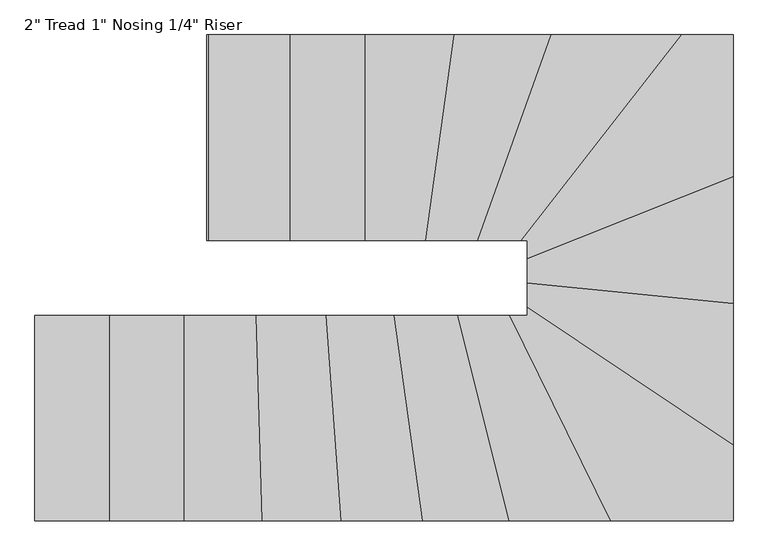
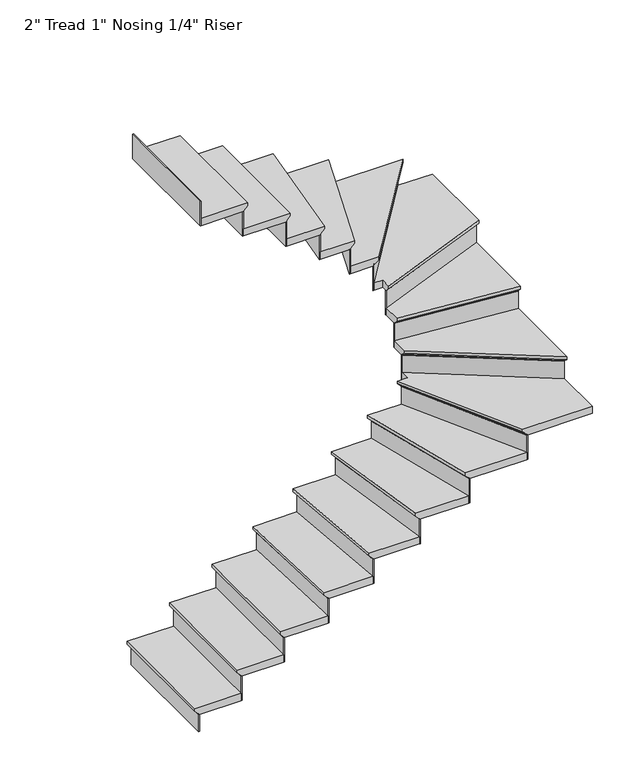
"""IFC4 building model written with IfcOpenShell, lengths in millimetres: stair flight geometry."""

from ifc_helpers import new_model, si_unit, origin, place, context, project, spatial, faceted_brep, source, transform, mapped, element, save


def stair_flight_f4c31f77(model_context):
    return source(origin(), model_context, "Body", "Brep", [
        faceted_brep([(-7679.0298583, 5178.9261204, 150.2833333), (-7679.0298583, 5178.9261204, 169.3333333), (-7679.0298583, 5948.2839473, 169.3333333), (-7679.0298583, 5948.2839473, 150.2833333), (-7653.6298583, 5178.9261204, 124.8833333), (-7653.6298583, 5948.2839473, 124.8833333), (-7374.2298583, 5178.9261204, 169.3333333), (-7374.2298583, 5948.2839473, 169.3333333), (-7653.6298583, 5948.2839473, 118.5333333), (-7374.2298583, 5948.2839473, 118.5333333), (-7374.2298583, 5178.9261204, 118.5333333), (-7653.6298583, 5178.9261204, 118.5333333)], [[[0, 1, 2, 3]], [[4, 0, 3, 5]], [[2, 1, 6, 7]], [[8, 9, 10, 11]], [[2, 7, 9, 8, 5, 3]], [[8, 11, 4, 5]], [[6, 1, 0, 4, 11, 10]], [[7, 6, 10, 9]]]),
        faceted_brep([(-7653.6298583, 5178.9261204, 118.5333333), (-7653.6298583, 5178.9261204, 0.0), (-7647.2798583, 5178.9261204, 0.0), (-7647.2798583, 5178.9261204, 118.5333333), (-7653.6298583, 5948.2839473, 118.5333333), (-7647.2798583, 5948.2839473, 118.5333333), (-7647.2798583, 5948.2839473, 0.0), (-7653.6298583, 5948.2839473, 0.0)], [[[0, 1, 2, 3]], [[4, 5, 6, 7]], [[1, 0, 4, 7]], [[2, 1, 7, 6]], [[3, 2, 6, 5]], [[0, 3, 5, 4]]]),
        faceted_brep([(-7374.2298583, 5178.9261204, 287.8666667), (-7374.2298583, 5178.9261204, 118.5333333), (-7367.8798583, 5178.9261204, 118.5333333), (-7367.8798583, 5178.9261204, 287.8666667), (-7374.2298583, 5948.2839473, 287.8666667), (-7367.8798583, 5948.2839473, 287.8666667), (-7367.8798583, 5948.2839473, 118.5333333), (-7374.2298583, 5948.2839473, 118.5333333)], [[[0, 1, 2, 3]], [[4, 5, 6, 7]], [[1, 0, 4, 7]], [[2, 1, 7, 6]], [[3, 2, 6, 5]], [[0, 3, 5, 4]]]),
        faceted_brep([(-7399.6298583, 5948.2839473, 338.6666667), (-7399.6298583, 5178.9261204, 338.6666667), (-7094.8298583, 5178.9261204, 338.6666667), (-7094.8298583, 5948.2839473, 338.6666667), (-7374.2298583, 5948.2839473, 287.8666667), (-7094.8298583, 5948.2839473, 287.8666667), (-7094.8298583, 5178.9261204, 287.8666667), (-7374.2298583, 5178.9261204, 287.8666667), (-7374.2298583, 5948.2839473, 294.2166667), (-7399.6298583, 5948.2839473, 319.6166667), (-7374.2298583, 5178.9261204, 294.2166667), (-7399.6298583, 5178.9261204, 319.6166667)], [[[0, 1, 2, 3]], [[4, 5, 6, 7]], [[0, 3, 5, 4, 8, 9]], [[4, 7, 10, 8]], [[2, 1, 11, 10, 7, 6]], [[3, 2, 6, 5]], [[11, 1, 0, 9]], [[10, 11, 9, 8]]]),
        faceted_brep([(-7094.8298583, 5178.9261204, 457.2), (-7094.8298583, 5178.9261204, 287.8666667), (-7088.4798583, 5178.9261204, 287.8666667), (-7088.4798583, 5178.9261204, 457.2), (-7094.8298583, 5948.2839473, 457.2), (-7088.4798583, 5948.2839473, 457.2), (-7088.4798583, 5948.2839473, 287.8666667), (-7094.8298583, 5948.2839473, 287.8666667)], [[[0, 1, 2, 3]], [[4, 5, 6, 7]], [[1, 0, 4, 7]], [[2, 1, 7, 6]], [[3, 2, 6, 5]], [[0, 3, 5, 4]]]),
        faceted_brep([(-7120.2298583, 5948.2839473, 508.0), (-7120.2298583, 5178.9261204, 508.0), (-6803.7593051, 5178.9261204, 508.0), (-6827.0770849, 5948.2839473, 508.0), (-7094.8298583, 5948.2839473, 457.2), (-6827.0770849, 5948.2839473, 457.2), (-6803.7593051, 5178.9261204, 457.2), (-7094.8298583, 5178.9261204, 457.2), (-7094.8298583, 5948.2839473, 463.55), (-7120.2298583, 5948.2839473, 488.95), (-7094.8298583, 5178.9261204, 463.55), (-7120.2298583, 5178.9261204, 488.95)], [[[0, 1, 2, 3]], [[4, 5, 6, 7]], [[0, 3, 5, 4, 8, 9]], [[4, 7, 10, 8]], [[2, 1, 11, 10, 7, 6]], [[3, 2, 6, 5]], [[11, 1, 0, 9]], [[10, 11, 9, 8]]]),
        faceted_brep([(-6803.7593051, 5178.9261204, 626.5333333), (-6803.7593051, 5178.9261204, 457.2), (-6797.4063893, 5178.9261204, 457.2), (-6797.4063893, 5178.9261204, 626.5333333), (-6827.0770849, 5948.2839473, 626.5333333), (-6820.7241691, 5948.2839473, 626.5333333), (-6820.7241691, 5948.2839473, 457.2), (-6827.0770849, 5948.2839473, 457.2)], [[[0, 1, 2, 3]], [[4, 5, 6, 7]], [[1, 0, 4, 7]], [[2, 1, 7, 6]], [[3, 2, 6, 5]], [[0, 3, 5, 4]]]),
        faceted_brep([(-6852.4887482, 5948.2839473, 677.3333333), (-6829.1709684, 5178.9261204, 677.3333333), (-6507.7862116, 5178.9261204, 677.3333333), (-6564.1374226, 5948.2839473, 677.3333333), (-6827.0770849, 5948.2839473, 626.5333333), (-6564.1374226, 5948.2839473, 626.5333333), (-6507.7862116, 5178.9261204, 626.5333333), (-6803.7593051, 5178.9261204, 626.5333333), (-6827.0770849, 5948.2839473, 632.8833333), (-6852.4887482, 5948.2839473, 658.2833333), (-6803.7593051, 5178.9261204, 632.8833333), (-6829.1709684, 5178.9261204, 658.2833333)], [[[0, 1, 2, 3]], [[4, 5, 6, 7]], [[0, 3, 5, 4, 8, 9]], [[4, 7, 10, 8]], [[2, 1, 11, 10, 7, 6]], [[3, 2, 6, 5]], [[11, 1, 0, 9]], [[10, 11, 9, 8]]]),
        faceted_brep([(-6507.7862116, 5178.9261204, 795.8666667), (-6507.7862116, 5178.9261204, 626.5333333), (-6501.4192013, 5178.9261204, 626.5333333), (-6501.4192013, 5178.9261204, 795.8666667), (-6564.1374226, 5948.2839473, 795.8666667), (-6557.7704123, 5948.2839473, 795.8666667), (-6557.7704123, 5948.2839473, 626.5333333), (-6564.1374226, 5948.2839473, 626.5333333)], [[[0, 1, 2, 3]], [[4, 5, 6, 7]], [[1, 0, 4, 7]], [[2, 1, 7, 6]], [[3, 2, 6, 5]], [[0, 3, 5, 4]]]),
        faceted_brep([(-6589.6054638, 5948.2839473, 846.6666667), (-6533.2542529, 5178.9261204, 846.6666667), (-6203.0012017, 5178.9261204, 846.6666667), (-6309.7716562, 5948.2839473, 846.6666667), (-6564.1374226, 5948.2839473, 795.8666667), (-6309.7716562, 5948.2839473, 795.8666667), (-6203.0012017, 5178.9261204, 795.8666667), (-6507.7862116, 5178.9261204, 795.8666667), (-6564.1374226, 5948.2839473, 802.2166667), (-6589.6054638, 5948.2839473, 827.6166667), (-6507.7862116, 5178.9261204, 802.2166667), (-6533.2542529, 5178.9261204, 827.6166667)], [[[0, 1, 2, 3]], [[4, 5, 6, 7]], [[0, 3, 5, 4, 8, 9]], [[4, 7, 10, 8]], [[2, 1, 11, 10, 7, 6]], [[3, 2, 6, 5]], [[11, 1, 0, 9]], [[10, 11, 9, 8]]]),
        faceted_brep([(-6203.0012017, 5178.9261204, 965.2), (-6203.0012017, 5178.9261204, 795.8666667), (-6196.5903443, 5178.9261204, 795.8666667), (-6196.5903443, 5178.9261204, 965.2), (-6309.7716562, 5948.2839473, 965.2), (-6303.3607989, 5948.2839473, 965.2), (-6303.3607989, 5948.2839473, 795.8666667), (-6309.7716562, 5948.2839473, 795.8666667)], [[[0, 1, 2, 3]], [[4, 5, 6, 7]], [[1, 0, 4, 7]], [[2, 1, 7, 6]], [[3, 2, 6, 5]], [[0, 3, 5, 4]]]),
        faceted_brep([(-6335.4150856, 5948.2839473, 1016.0), (-6228.6446311, 5178.9261204, 1016.0), (-5879.8397743, 5178.9261204, 1016.0), (-6073.0426446, 5948.2839473, 1016.0), (-6309.7716562, 5948.2839473, 965.2), (-6073.0426446, 5948.2839473, 965.2), (-5879.8397743, 5178.9261204, 965.2), (-6203.0012017, 5178.9261204, 965.2), (-6309.7716562, 5948.2839473, 971.55), (-6335.4150856, 5948.2839473, 996.95), (-6203.0012017, 5178.9261204, 971.55), (-6228.6446311, 5178.9261204, 996.95)], [[[0, 1, 2, 3]], [[4, 5, 6, 7]], [[0, 3, 5, 4, 8, 9]], [[4, 7, 10, 8]], [[2, 1, 11, 10, 7, 6]], [[3, 2, 6, 5]], [[11, 1, 0, 9]], [[10, 11, 9, 8]]]),
        faceted_brep([(-5879.8397743, 5178.9261204, 1134.5333333), (-5879.8397743, 5178.9261204, 965.2), (-5873.2926121, 5178.9261204, 965.2), (-5873.2926121, 5178.9261204, 1134.5333333), (-6073.0426446, 5948.2839473, 1134.5333333), (-6066.4954824, 5948.2839473, 1134.5333333), (-6066.4954824, 5948.2839473, 965.2), (-6073.0426446, 5948.2839473, 965.2)], [[[0, 1, 2, 3]], [[4, 5, 6, 7]], [[1, 0, 4, 7]], [[2, 1, 7, 6]], [[3, 2, 6, 5]], [[0, 3, 5, 4]]]),
        faceted_brep([(-6099.2312935, 5948.2839473, 1185.3333333), (-5906.0284232, 5178.9261204, 1185.3333333), (-5497.940126, 5178.9261204, 1185.3333333), (-5875.7797358, 5948.2839473, 1185.3333333), (-6073.0426446, 5948.2839473, 1134.5333333), (-5875.7797358, 5948.2839473, 1134.5333333), (-5497.940126, 5178.9261204, 1134.5333333), (-5879.8397743, 5178.9261204, 1134.5333333), (-6073.0426446, 5948.2839473, 1140.8833333), (-6099.2312935, 5948.2839473, 1166.2833333), (-5879.8397743, 5178.9261204, 1140.8833333), (-5906.0284232, 5178.9261204, 1166.2833333)], [[[0, 1, 2, 3]], [[4, 5, 6, 7]], [[0, 3, 5, 4, 8, 9]], [[4, 7, 10, 8]], [[2, 1, 11, 10, 7, 6]], [[3, 2, 6, 5]], [[11, 1, 0, 9]], [[10, 11, 9, 8]]]),
        faceted_brep([(-5497.940126, 5178.9261204, 1303.8666667), (-5497.940126, 5178.9261204, 1134.5333333), (-5490.8656748, 5178.9261204, 1134.5333333), (-5490.8656748, 5178.9261204, 1303.8666667), (-5875.7797358, 5948.2839473, 1303.8666667), (-5868.7052846, 5948.2839473, 1303.8666667), (-5868.7052846, 5948.2839473, 1134.5333333), (-5875.7797358, 5948.2839473, 1134.5333333)], [[[0, 1, 2, 3]], [[4, 5, 6, 7]], [[1, 0, 4, 7]], [[2, 1, 7, 6]], [[3, 2, 6, 5]], [[0, 3, 5, 4]]]),
        faceted_brep([(-5838.68475, 6008.9671044, 1354.6666667), (-5838.68475, 5948.2839473, 1354.6666667), (-5904.0775406, 5948.2839473, 1354.6666667), (-5526.2379307, 5178.9261204, 1354.6666667), (-5069.3269231, 5178.9261204, 1354.6666667), (-5069.3269231, 5494.6042749, 1354.6666667), (-5838.68475, 5948.2839473, 1303.8666667), (-5838.68475, 6008.9671044, 1303.8666667), (-5069.3269231, 5494.6042749, 1303.8666667), (-5069.3269231, 5178.9261204, 1303.8666667), (-5497.940126, 5178.9261204, 1303.8666667), (-5875.7797358, 5948.2839473, 1303.8666667), (-5497.940126, 5178.9261204, 1310.2166667), (-5875.7797358, 5948.2839473, 1310.2166667), (-5526.2379307, 5178.9261204, 1335.6166667), (-5904.0775406, 5948.2839473, 1335.6166667)], [[[0, 1, 2, 3, 4, 5]], [[6, 7, 8, 9, 10, 11]], [[1, 0, 7, 6]], [[11, 10, 12, 13]], [[5, 4, 9, 8]], [[0, 5, 8, 7]], [[14, 3, 2, 15]], [[12, 14, 15, 13]], [[4, 3, 14, 12, 10, 9]], [[2, 1, 6, 11, 13, 15]]]),
        faceted_brep([(-5069.3269231, 5494.6042749, 1473.2), (-5069.3269231, 5494.6042749, 1303.8666667), (-5069.3269231, 5502.242705, 1303.8666667), (-5069.3269231, 5502.242705, 1473.2), (-5838.68475, 6008.9671044, 1473.2), (-5838.68475, 6016.6055346, 1473.2), (-5838.68475, 6016.6055346, 1303.8666667), (-5838.68475, 6008.9671044, 1303.8666667)], [[[0, 1, 2, 3]], [[4, 5, 6, 7]], [[1, 0, 4, 7]], [[2, 1, 7, 6]], [[3, 2, 6, 5]], [[0, 3, 5, 4]]]),
        faceted_brep([(-5838.68475, 5978.4133839, 1524.0), (-5069.3269231, 5464.0505544, 1524.0), (-5069.3269231, 6017.5402175, 1524.0), (-5838.68475, 6094.2010538, 1524.0), (-5838.68475, 6008.9671044, 1473.2), (-5838.68475, 6094.2010538, 1473.2), (-5069.3269231, 6017.5402175, 1473.2), (-5069.3269231, 5494.6042749, 1473.2), (-5838.68475, 6008.9671044, 1479.55), (-5838.68475, 5978.4133839, 1504.95), (-5069.3269231, 5494.6042749, 1479.55), (-5069.3269231, 5464.0505544, 1504.95)], [[[0, 1, 2, 3]], [[4, 5, 6, 7]], [[0, 3, 5, 4, 8, 9]], [[4, 7, 10, 8]], [[2, 1, 11, 10, 7, 6]], [[3, 2, 6, 5]], [[11, 1, 0, 9]], [[10, 11, 9, 8]]]),
        faceted_brep([(-5069.3269231, 6017.5402175, 1642.5333333), (-5069.3269231, 6017.5402175, 1473.2), (-5069.3269231, 6023.9216631, 1473.2), (-5069.3269231, 6023.9216631, 1642.5333333), (-5838.68475, 6094.2010538, 1642.5333333), (-5838.68475, 6100.5824994, 1642.5333333), (-5838.68475, 6100.5824994, 1473.2), (-5838.68475, 6094.2010538, 1473.2)], [[[0, 1, 2, 3]], [[4, 5, 6, 7]], [[1, 0, 4, 7]], [[2, 1, 7, 6]], [[3, 2, 6, 5]], [[0, 3, 5, 4]]]),
        faceted_brep([(-5838.68475, 6068.6752714, 1693.3333333), (-5069.3269231, 5992.014435, 1693.3333333), (-5069.3269231, 6493.5749269, 1693.3333333), (-5838.68475, 6187.3373104, 1693.3333333), (-5838.68475, 6094.2010538, 1642.5333333), (-5838.68475, 6187.3373104, 1642.5333333), (-5069.3269231, 6493.5749269, 1642.5333333), (-5069.3269231, 6017.5402175, 1642.5333333), (-5838.68475, 6094.2010538, 1648.8833333), (-5838.68475, 6068.6752714, 1674.2833333), (-5069.3269231, 6017.5402175, 1648.8833333), (-5069.3269231, 5992.014435, 1674.2833333)], [[[0, 1, 2, 3]], [[4, 5, 6, 7]], [[0, 3, 5, 4, 8, 9]], [[4, 7, 10, 8]], [[2, 1, 11, 10, 7, 6]], [[3, 2, 6, 5]], [[11, 1, 0, 9]], [[10, 11, 9, 8]]]),
        faceted_brep([(-5069.3269231, 6493.5749269, 1811.8666667), (-5069.3269231, 6493.5749269, 1642.5333333), (-5069.3269231, 6500.4094811, 1642.5333333), (-5069.3269231, 6500.4094811, 1811.8666667), (-5838.68475, 6187.3373104, 1811.8666667), (-5838.68475, 6194.1718646, 1811.8666667), (-5838.68475, 6194.1718646, 1642.5333333), (-5838.68475, 6187.3373104, 1642.5333333)], [[[0, 1, 2, 3]], [[4, 5, 6, 7]], [[1, 0, 4, 7]], [[2, 1, 7, 6]], [[3, 2, 6, 5]], [[0, 3, 5, 4]]]),
        faceted_brep([(-5895.4681858, 6227.6839473, 1862.6666667), (-5838.68475, 6227.6839473, 1862.6666667), (-5838.68475, 6159.9990938, 1862.6666667), (-5069.3269231, 6466.2367103, 1862.6666667), (-5069.3269231, 6997.0417743, 1862.6666667), (-5294.4198376, 6997.0417743, 1862.6666667), (-5838.68475, 6227.6839473, 1811.8666667), (-5895.4681858, 6227.6839473, 1811.8666667), (-5294.4198376, 6997.0417743, 1811.8666667), (-5069.3269231, 6997.0417743, 1811.8666667), (-5069.3269231, 6493.5749269, 1811.8666667), (-5838.68475, 6187.3373104, 1811.8666667), (-5838.68475, 6187.3373104, 1818.2166667), (-5838.68475, 6159.9990938, 1843.6166667), (-5069.3269231, 6493.5749269, 1818.2166667), (-5069.3269231, 6466.2367103, 1843.6166667)], [[[0, 1, 2, 3, 4, 5]], [[6, 7, 8, 9, 10, 11]], [[1, 0, 7, 6]], [[2, 1, 6, 11, 12, 13]], [[11, 10, 14, 12]], [[4, 3, 15, 14, 10, 9]], [[0, 5, 8, 7]], [[15, 3, 2, 13]], [[14, 15, 13, 12]], [[5, 4, 9, 8]]]),
        faceted_brep([(-5294.4198376, 6997.0417743, 1981.2), (-5294.4198376, 6997.0417743, 1811.8666667), (-5302.4779007, 6997.0417743, 1811.8666667), (-5302.4779007, 6997.0417743, 1981.2), (-5895.4681858, 6227.6839473, 1981.2), (-5903.5262489, 6227.6839473, 1981.2), (-5903.5262489, 6227.6839473, 1811.8666667), (-5895.4681858, 6227.6839473, 1811.8666667)], [[[0, 1, 2, 3]], [[4, 5, 6, 7]], [[1, 0, 4, 7]], [[2, 1, 7, 6]], [[3, 2, 6, 5]], [[0, 3, 5, 4]]]),
        faceted_brep([(-5863.2359334, 6227.6839473, 2032.0), (-5262.1875852, 6997.0417743, 2032.0), (-5777.8246211, 6997.0417743, 2032.0), (-6051.8904456, 6227.6839473, 2032.0), (-5895.4681858, 6227.6839473, 1981.2), (-6051.8904456, 6227.6839473, 1981.2), (-5777.8246211, 6997.0417743, 1981.2), (-5294.4198376, 6997.0417743, 1981.2), (-5895.4681858, 6227.6839473, 1987.55), (-5863.2359334, 6227.6839473, 2012.95), (-5294.4198376, 6997.0417743, 1987.55), (-5262.1875852, 6997.0417743, 2012.95)], [[[0, 1, 2, 3]], [[4, 5, 6, 7]], [[0, 3, 5, 4, 8, 9]], [[4, 7, 10, 8]], [[2, 1, 11, 10, 7, 6]], [[3, 2, 6, 5]], [[11, 1, 0, 9]], [[10, 11, 9, 8]]]),
        faceted_brep([(-5777.8246211, 6997.0417743, 2150.5333333), (-5777.8246211, 6997.0417743, 1981.2), (-5784.5654908, 6997.0417743, 1981.2), (-5784.5654908, 6997.0417743, 2150.5333333), (-6051.8904456, 6227.6839473, 2150.5333333), (-6058.6313153, 6227.6839473, 2150.5333333), (-6058.6313153, 6227.6839473, 1981.2), (-6051.8904456, 6227.6839473, 1981.2)], [[[0, 1, 2, 3]], [[4, 5, 6, 7]], [[1, 0, 4, 7]], [[2, 1, 7, 6]], [[3, 2, 6, 5]], [[0, 3, 5, 4]]]),
        faceted_brep([(-6024.9269669, 6227.6839473, 2201.3333333), (-5750.8611424, 6997.0417743, 2201.3333333), (-6139.3552274, 6997.0417743, 2201.3333333), (-6246.5233568, 6227.6839473, 2201.3333333), (-6051.8904456, 6227.6839473, 2150.5333333), (-6246.5233568, 6227.6839473, 2150.5333333), (-6139.3552274, 6997.0417743, 2150.5333333), (-5777.8246211, 6997.0417743, 2150.5333333), (-6051.8904456, 6227.6839473, 2156.8833333), (-6024.9269669, 6227.6839473, 2182.2833333), (-5777.8246211, 6997.0417743, 2156.8833333), (-5750.8611424, 6997.0417743, 2182.2833333)], [[[0, 1, 2, 3]], [[4, 5, 6, 7]], [[0, 3, 5, 4, 8, 9]], [[4, 7, 10, 8]], [[2, 1, 11, 10, 7, 6]], [[3, 2, 6, 5]], [[11, 1, 0, 9]], [[10, 11, 9, 8]]]),
        faceted_brep([(-6139.3552274, 6997.0417743, 2319.8666667), (-6139.3552274, 6997.0417743, 2150.5333333), (-6145.7665368, 6997.0417743, 2150.5333333), (-6145.7665368, 6997.0417743, 2319.8666667), (-6246.5233568, 6227.6839473, 2319.8666667), (-6252.9346661, 6227.6839473, 2319.8666667), (-6252.9346661, 6227.6839473, 2150.5333333), (-6246.5233568, 6227.6839473, 2150.5333333)], [[[0, 1, 2, 3]], [[4, 5, 6, 7]], [[1, 0, 4, 7]], [[2, 1, 7, 6]], [[3, 2, 6, 5]], [[0, 3, 5, 4]]]),
        faceted_brep([(-6220.8781194, 6227.6839473, 2370.6666667), (-6113.70999, 6997.0417743, 2370.6666667), (-6472.0940547, 6997.0417743, 2370.6666667), (-6472.0940547, 6227.6839473, 2370.6666667), (-6246.5233568, 6227.6839473, 2319.8666667), (-6472.0940547, 6227.6839473, 2319.8666667), (-6472.0940547, 6997.0417743, 2319.8666667), (-6139.3552274, 6997.0417743, 2319.8666667), (-6246.5233568, 6227.6839473, 2326.2166667), (-6220.8781194, 6227.6839473, 2351.6166667), (-6139.3552274, 6997.0417743, 2326.2166667), (-6113.70999, 6997.0417743, 2351.6166667)], [[[0, 1, 2, 3]], [[4, 5, 6, 7]], [[0, 3, 5, 4, 8, 9]], [[4, 7, 10, 8]], [[2, 1, 11, 10, 7, 6]], [[3, 2, 6, 5]], [[11, 1, 0, 9]], [[10, 11, 9, 8]]]),
        faceted_brep([(-6472.0940547, 6997.0417743, 2489.2), (-6472.0940547, 6997.0417743, 2319.8666667), (-6478.4440547, 6997.0417743, 2319.8666667), (-6478.4440547, 6997.0417743, 2489.2), (-6472.0940547, 6227.6839473, 2489.2), (-6478.4440547, 6227.6839473, 2489.2), (-6478.4440547, 6227.6839473, 2319.8666667), (-6472.0940547, 6227.6839473, 2319.8666667)], [[[0, 1, 2, 3]], [[4, 5, 6, 7]], [[1, 0, 4, 7]], [[2, 1, 7, 6]], [[3, 2, 6, 5]], [[0, 3, 5, 4]]]),
        faceted_brep([(-6446.6940547, 6227.6839473, 2540.0), (-6446.6940547, 6997.0417743, 2540.0), (-6751.4940547, 6997.0417743, 2540.0), (-6751.4940547, 6227.6839473, 2540.0), (-6472.0940547, 6227.6839473, 2489.2), (-6751.4940547, 6227.6839473, 2489.2), (-6751.4940547, 6997.0417743, 2489.2), (-6472.0940547, 6997.0417743, 2489.2), (-6472.0940547, 6227.6839473, 2495.55), (-6446.6940547, 6227.6839473, 2520.95), (-6472.0940547, 6997.0417743, 2495.55), (-6446.6940547, 6997.0417743, 2520.95)], [[[0, 1, 2, 3]], [[4, 5, 6, 7]], [[0, 3, 5, 4, 8, 9]], [[4, 7, 10, 8]], [[2, 1, 11, 10, 7, 6]], [[3, 2, 6, 5]], [[11, 1, 0, 9]], [[10, 11, 9, 8]]]),
        faceted_brep([(-6751.4940547, 6997.0417743, 2658.5333333), (-6751.4940547, 6997.0417743, 2489.2), (-6757.8440547, 6997.0417743, 2489.2), (-6757.8440547, 6997.0417743, 2658.5333333), (-6751.4940547, 6227.6839473, 2658.5333333), (-6757.8440547, 6227.6839473, 2658.5333333), (-6757.8440547, 6227.6839473, 2489.2), (-6751.4940547, 6227.6839473, 2489.2)], [[[0, 1, 2, 3]], [[4, 5, 6, 7]], [[1, 0, 4, 7]], [[2, 1, 7, 6]], [[3, 2, 6, 5]], [[0, 3, 5, 4]]]),
        faceted_brep([(-7030.8940547, 6997.0417743, 2827.8666667), (-7030.8940547, 6997.0417743, 2658.5333333), (-7037.2440547, 6997.0417743, 2658.5333333), (-7037.2440547, 6997.0417743, 2827.8666667), (-7030.8940547, 6227.6839473, 2827.8666667), (-7037.2440547, 6227.6839473, 2827.8666667), (-7037.2440547, 6227.6839473, 2658.5333333), (-7030.8940547, 6227.6839473, 2658.5333333)], [[[0, 1, 2, 3]], [[4, 5, 6, 7]], [[1, 0, 4, 7]], [[2, 1, 7, 6]], [[3, 2, 6, 5]], [[0, 3, 5, 4]]]),
        faceted_brep([(-6726.0940547, 6227.6839473, 2709.3333333), (-6726.0940547, 6997.0417743, 2709.3333333), (-7030.8940547, 6997.0417743, 2709.3333333), (-7030.8940547, 6227.6839473, 2709.3333333), (-6751.4940547, 6227.6839473, 2658.5333333), (-7030.8940547, 6227.6839473, 2658.5333333), (-7030.8940547, 6997.0417743, 2658.5333333), (-6751.4940547, 6997.0417743, 2658.5333333), (-6751.4940547, 6227.6839473, 2664.8833333), (-6726.0940547, 6227.6839473, 2690.2833333), (-6751.4940547, 6997.0417743, 2664.8833333), (-6726.0940547, 6997.0417743, 2690.2833333)], [[[0, 1, 2, 3]], [[4, 5, 6, 7]], [[0, 3, 5, 4, 8, 9]], [[4, 7, 10, 8]], [[2, 1, 11, 10, 7, 6]], [[3, 2, 6, 5]], [[11, 1, 0, 9]], [[10, 11, 9, 8]]]),
    ])


if __name__ == "__main__":
    model = new_model("IFC4")
    model_context = context("Model", 3, world=origin())
    ifc_project = project(units=[si_unit("LENGTHUNIT", "METRE", prefix="MILLI")], contexts=[model_context])
    site = spatial("IfcSite", under=ifc_project)
    building = spatial("IfcBuilding", under=site)
    placement = place(None, origin())
    stair_flight_shape = stair_flight_f4c31f77(model_context)
    element("IfcStairFlight", 1, ObjectType="2\" Tread 1\" Nosing 1/4\" Riser", at=placement, inside=building, context=model_context, shape_type="MappedRepresentation", body=[
        mapped(stair_flight_shape, transform((0.0, 0.0, 0.0), x_axis=(1.0, 0.0, 0.0), y_axis=(0.0, 1.0, 0.0), z_axis=(0.0, 0.0, 1.0))),
    ])
    save(model, "model.ifc")
